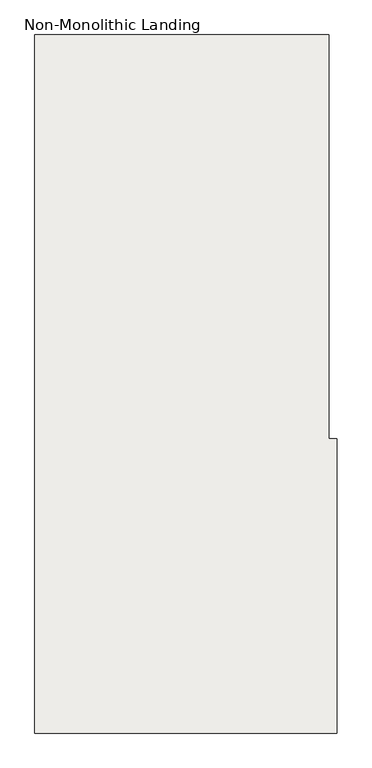
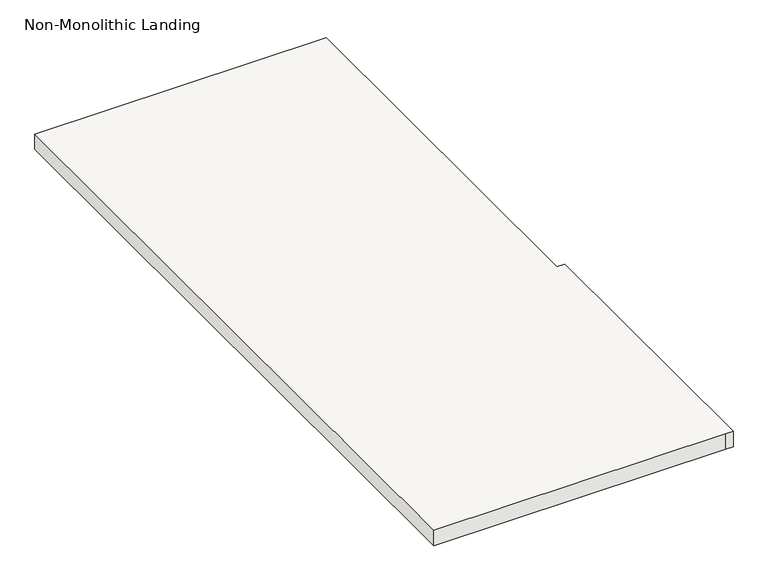
"""IFC4 building model written with IfcOpenShell, lengths in millimetres: slab geometry, Non-Monolithic Landing."""

from ifc_helpers import new_model, si_unit, origin, place, context, project, spatial, faceted_brep, source, transform, mapped, element, save


def non_monolithic_landing_d7d9d8c2(model_context):
    return source(origin(), model_context, "Body", "Brep", [
        faceted_brep([(-12083.8120641, -2647.9669819, 2343.15), (-12058.4120641, -2647.9669819, 2368.55), (-12058.4120641, -3562.3669819, 2368.55), (-12083.8120641, -3562.3669819, 2343.15), (-12972.8120641, -2647.9669819, 2387.6), (-12972.8120641, -4817.9038196, 2387.6), (-12058.4120641, -4817.9038196, 2387.6), (-12033.0120641, -4817.9038196, 2387.6), (-12033.0120641, -3903.5038196, 2387.6), (-12058.4120641, -3903.5038196, 2387.6), (-12058.4120641, -2647.9669819, 2387.6), (-12083.8120641, -3562.3669819, 2336.8), (-12058.4120641, -3562.3669819, 2336.8), (-12058.4120641, -3903.5038196, 2336.8), (-12033.0120641, -3903.5038196, 2336.8), (-12033.0120641, -4817.9038196, 2336.8), (-12058.4120641, -4817.9038196, 2336.8), (-12972.8120641, -4817.9038196, 2336.8), (-12972.8120641, -2647.9669819, 2336.8), (-12083.8120641, -2647.9669819, 2336.8)], [[[0, 1, 2, 3]], [[4, 5, 6, 7, 8, 9, 10]], [[11, 12, 13, 14, 15, 16, 17, 18, 19]], [[12, 11, 3, 2]], [[11, 19, 0, 3]], [[4, 10, 1, 0, 19, 18]], [[5, 4, 18, 17]], [[6, 5, 17, 16]], [[7, 6, 16, 15]], [[8, 7, 15, 14]], [[9, 8, 14, 13]], [[10, 9, 13, 12, 2, 1]]]),
    ])


if __name__ == "__main__":
    model = new_model("IFC4")
    model_context = context("Model", 3, world=origin())
    ifc_project = project(units=[si_unit("LENGTHUNIT", "METRE", prefix="MILLI")], contexts=[model_context])
    site = spatial("IfcSite", under=ifc_project)
    building = spatial("IfcBuilding", under=site)
    placement = place(None, origin())
    non_monolithic_landing_shape = non_monolithic_landing_d7d9d8c2(model_context)
    element("IfcSlab", 1, ObjectType="Non-Monolithic Landing", at=placement, inside=building, context=model_context, shape_type="MappedRepresentation", body=[
        mapped(non_monolithic_landing_shape, transform((0.0, 0.0, 0.0), x_axis=(1.0, 0.0, 0.0), y_axis=(0.0, 1.0, 0.0), z_axis=(0.0, 0.0, 1.0))),
    ])
    save(model, "model.ifc")
